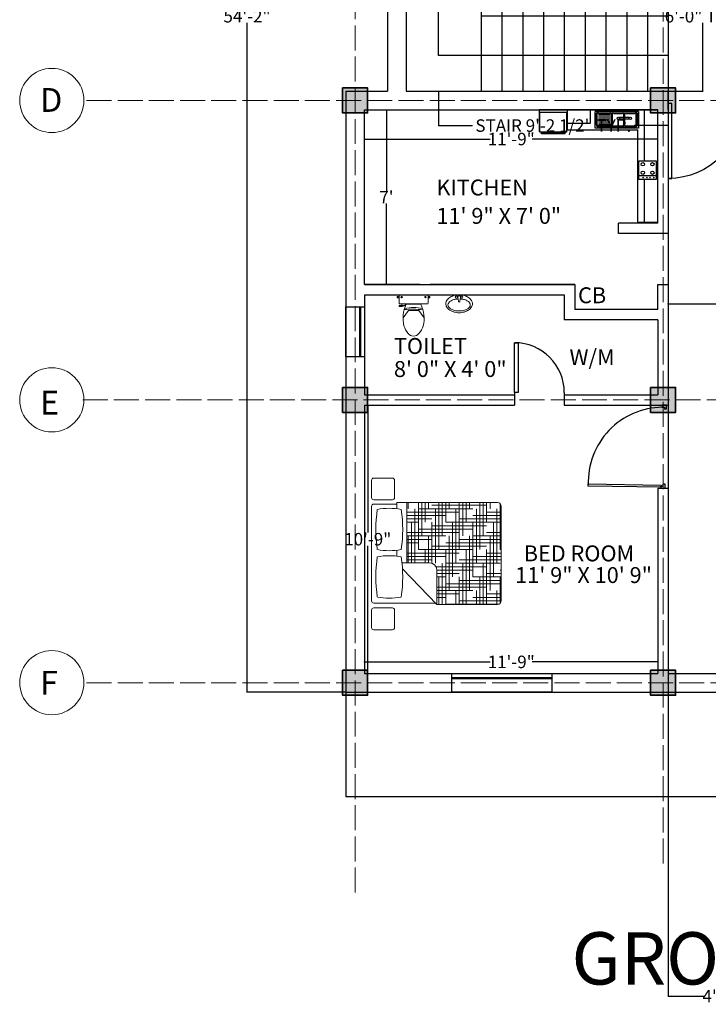
# Model space of a CAD drawing. Units: inches. Extents: x -113 to 5399, y -1393 to 3302.
# Tile 2 of 40: x 737 to 1068, y -14 to 460. Entities that reach past the tile are written whole.
import ezdxf

# ---------------------------------------------------------------- set-up
doc = ezdxf.new("R2010")
doc.units = ezdxf.units.IN
doc.header["$MEASUREMENT"] = 0
doc.linetypes.add('ACAD_ISO02W100', pattern=[15, 12, -3])
for name, color, linetype, lineweight in [('A-ANNO-DIMS', 254, 'Continuous', 18), ('A-ANNO-TEXT', 7, 'Continuous', 25), ('A-AREA-IDEN', 4, 'Continuous', 18), ('A-COLS', 7, 'Continuous', 35), ('A-FLOR-CASE', 8, 'Continuous', 18), ('A-FLOR-FIXT', 8, 'Continuous', 18), ('A-GRID-IDEN', 7, 'Continuous', 18), ('doors', 2, 'Continuous', 25), ('DT TEXT', 4, 'Continuous', 18), ('furniture', 131, 'Continuous', 18), ('GRIDS', 7, 'ACAD_ISO02W100', 13), ('stairs', 210, 'Continuous', 25), ('walls', 1, 'Continuous', 25), ('windows', 3, 'Continuous', 25)]:
    doc.layers.add(name, color=color, linetype=linetype, lineweight=lineweight)
doc.layers.add('TEFRIŞ', color=11, linetype='Continuous')
doc.styles.get("Standard").update_dxf_attribs({"font": 'arial.ttf'})
doc.dimstyles.get("Standard").update_dxf_attribs({"dimtxt": 6, "dimasz": 0.18, "dimexe": 0.18, "dimexo": 0.0625, "dimgap": 0.09, "dimtad": 0, "dimtih": 1, "dimtoh": 1, "dimdec": 1, "dimzin": 0, "dimdsep": 46, "dimlunit": 4, "dimtxsty": 'Standard', "dimblk": 'ARCHTICK', "dimcen": 0.09, "dimadec": 0, "dimazin": 0, "dimtfac": 1, "dimtdec": 1, "dimtofl": 0, "dimtmove": 0, "dimatfit": 3, "dimfxl": 1, "dimtolj": 1, "dimtzin": 0, "dimarcsym": 0})

# ---------------------------------------------------------------- blocks, each defined once
blk = doc.blocks.new('*U2')
for p, q in [((0, 0), (0, -6)), ((24, 0), (24, -6))]:
    blk.add_line(p, q)
blk.add_lwpolyline([(0, 0), (0, 24), (1.75, 24), (1.75, 0)], close=True)
blk.add_arc((0, 0), 24, 0, 90)
blk = doc.blocks.new('*U3')
for p, q in [((0, 0), (0, -6)), ((36, 0), (36, -6))]:
    blk.add_line(p, q)
blk.add_lwpolyline([(0, 0), (0, 36), (1.75, 36), (1.75, 0)], close=True)
blk.add_arc((0, 0), 36, 0, 90)
blk = doc.blocks.new('*X4')
at = {"color": 0}
for p, q in [((4.359, 18.562), (4.359, 18.646)), ((4.453, 17.817), (4.453, 18.562)), ((4.5, 18), (4.5, 18.646)), ((4.5, 18.562), (5.25, 18.562)), ((4.547, 18.188), (4.547, 18.646)), ((4.594, 18.375), (4.594, 18.646)), ((4.641, 18.562), (4.641, 18.646)), ((4.687, 18.609), (5.437, 18.609)), ((4.734, 17.812), (4.734, 18.562)), ((4.781, 18), (4.781, 18.646)), ((4.828, 18.188), (4.828, 18.646)), ((4.875, 18.375), (4.875, 18.646)), ((4.922, 18.562), (4.922, 18.646)), ((5.016, 17.812), (5.016, 18.562)), ((5.062, 18), (5.062, 18.646)), ((5.109, 18.188), (5.109, 18.646)), ((5.156, 18.375), (5.156, 18.646)), ((5.203, 18.562), (5.203, 18.646)), ((5.297, 17.812), (5.297, 18.562)), ((5.344, 18), (5.344, 18.646)), ((5.391, 18.188), (5.391, 18.646)), ((5.437, 18.375), (5.437, 18.646)), ((5.484, 18.562), (5.484, 18.646)), ((5.578, 17.812), (5.578, 18.562)), ((5.625, 18), (5.625, 18.629)), ((5.625, 18.562), (5.637, 18.562)), ((4.34, 18.516), (5.062, 18.516)), ((4.34, 18.469), (4.875, 18.469)), ((4.34, 18.422), (4.687, 18.422)), ((5.062, 18.422), (5.637, 18.422)), ((5.25, 18.469), (5.637, 18.469)), ((5.437, 18.516), (5.637, 18.516)), ((4.34, 18.375), (4.5, 18.375)), ((4.406, 17.817), (4.406, 18.375)), ((4.5, 18.281), (5.25, 18.281)), ((4.687, 18.328), (5.437, 18.328)), ((4.687, 17.811), (4.687, 18.375)), ((4.875, 18.375), (5.625, 18.375)), ((4.969, 17.625), (4.969, 18.375)), ((5.25, 17.625), (5.25, 18.375)), ((5.531, 17.625), (5.531, 18.375)), ((5.625, 18.281), (5.637, 18.281)), ((4.34, 18.234), (5.062, 18.234)), ((4.34, 18.188), (4.875, 18.188)), ((4.34, 18.141), (4.687, 18.141)), ((4.359, 17.817), (4.359, 18.188)), ((4.641, 17.817), (4.641, 18.188)), ((4.922, 17.438), (4.922, 18.188)), ((5.062, 18.141), (5.637, 18.141)), ((5.203, 17.438), (5.203, 18.188)), ((5.25, 18.188), (5.637, 18.188)), ((5.437, 18.234), (5.637, 18.234)), ((5.484, 17.438), (5.484, 18.188)), ((4.34, 18.094), (4.5, 18.094)), ((4.5, 18), (5.25, 18)), ((4.594, 17.817), (4.594, 18)), ((4.687, 18.047), (5.437, 18.047)), ((4.875, 18.094), (5.625, 18.094)), ((4.875, 17.25), (4.875, 18)), ((5.156, 17.25), (5.156, 18)), ((5.437, 17.25), (5.437, 18)), ((5.625, 18), (5.637, 18)), ((4.34, 17.953), (5.062, 17.953)), ((4.34, 17.906), (4.875, 17.906)), ((4.34, 17.859), (4.687, 17.859)), ((5.062, 17.859), (5.637, 17.859)), ((5.25, 17.906), (5.637, 17.906)), ((5.437, 17.953), (5.637, 17.953)), ((4.742, 17.766), (5.437, 17.766)), ((4.755, 17.719), (5.25, 17.719)), ((4.828, 17.246), (4.828, 17.812)), ((4.875, 17.812), (5.625, 17.812)), ((5.109, 17.246), (5.109, 17.812)), ((5.391, 17.246), (5.391, 17.812)), ((5.625, 17.719), (5.637, 17.719)), ((4.755, 17.672), (5.062, 17.672)), ((4.755, 17.625), (4.875, 17.625)), ((4.781, 17.246), (4.781, 17.625)), ((5.062, 17.246), (5.062, 17.625)), ((5.062, 17.578), (5.637, 17.578)), ((5.25, 17.625), (5.637, 17.625)), ((5.344, 17.246), (5.344, 17.625)), ((5.437, 17.672), (5.637, 17.672)), ((5.625, 17.263), (5.625, 17.625)), ((4.755, 17.484), (5.437, 17.484)), ((4.875, 17.531), (5.625, 17.531)), ((4.755, 17.438), (5.25, 17.438)), ((4.755, 17.391), (5.062, 17.391)), ((4.755, 17.344), (4.875, 17.344)), ((5.016, 17.246), (5.016, 17.438)), ((5.25, 17.344), (5.637, 17.344)), ((5.297, 17.246), (5.297, 17.438)), ((5.437, 17.391), (5.637, 17.391)), ((5.578, 17.246), (5.578, 17.438)), ((5.625, 17.438), (5.637, 17.438)), ((4.875, 17.25), (5.608, 17.25)), ((4.969, 17.246), (4.969, 17.25)), ((5.062, 17.297), (5.637, 17.297)), ((5.25, 17.246), (5.25, 17.25)), ((5.531, 17.246), (5.531, 17.25))]:
    blk.add_line(p, q, dxfattribs=at)
blk = doc.blocks.new('MAT-P01')
for p, q in [((-0.021, 0.816), (-0.021, 0.56)), ((0.009, 0.846), (0.247, 0.846)), ((0.277, 0.816), (0.277, 0.56)), ((0.344, 0.816), (0.344, -0.032)), ((0.374, 0.846), (1.674, 0.846)), ((1.704, 0.816), (1.704, 0.5)), ((1.762, 0.816), (1.762, 0.56)), ((1.792, 0.846), (2.031, 0.846)), ((2.061, 0.816), (2.061, 0.56)), ((0.009, 0.53), (0.247, 0.53)), ((0.815, 0.423), (0.324, -0.051)), ((0.895, 0.429), (0.895, 0.049)), ((0.988, 0.5), (1.069, 0.5)), ((1.639, 0.5), (1.724, 0.5)), ((1.724, 0.5), (1.724, -0.884)), ((1.792, 0.53), (2.031, 0.53)), ((0.895, 0.364), (1.724, 0.364)), ((0.895, 0.364), (0.895, 0.049)), ((0.895, 0.364), (1.724, 0.364)), ((1.724, 0.364), (1.724, -0.884)), ((0.324, -0.051), (0.795, -0.051)), ((0.324, -0.051), (0.324, -0.884)), ((0.374, -0.934), (1.674, -0.934))]:
    blk.add_line(p, q)
for centre, radius, start, end in [((0.009, 0.816), 0.03, 90, 180), ((0.247, 0.816), 0.03, 0, 90), ((0.374, 0.816), 0.03, 90, 180), ((1.674, 0.816), 0.03, 0, 90), ((1.792, 0.816), 0.03, 90, 180), ((2.031, 0.816), 0.03, 0, 90), ((1.225, 0.603), 0.814, 168.373, 191.627), ((0.703, -1.144), 1.931, 81.8162, 98.1838), ((0.181, 0.603), 0.814, 348.373, 11.627), ((1.877, 0.603), 0.814, 168.373, 191.627), ((1.354, -1.144), 1.931, 81.8162, 98.1838), ((0.832, 0.603), 0.814, 348.373, 11.627), ((0.009, 0.56), 0.03, 180, 270), ((0.247, 0.56), 0.03, 270, 0), ((1.792, 0.56), 0.03, 180, 270), ((2.031, 0.56), 0.03, 270, 0), ((0.703, 2.35), 1.931, 261.8162, 278.1838), ((1.354, 2.35), 1.931, 261.8162, 278.1838), ((0.795, 0.049), 0.1, 270, 0), ((0.374, -0.884), 0.05, 180, 270), ((1.674, -0.884), 0.05, 270, 0)]:
    blk.add_arc(centre, radius, start, end)
at = {"rotation": 270}
blk.add_blockref('*X4', (-16.922, 4.704), dxfattribs=at)
blk = doc.blocks.new('A$C008029BD')
at = {"layer": 'TEFRIŞ', "ltscale": 0.05}
for p, q in [((0, 0), (0, -3.55)), ((3.37, 0), (0, 0)), ((3.37, 0), (3.37, -0.6)), ((1.522, -0.4), (0, -0.4)), ((0.05, -0.581), (0.05, -1.869)), ((0.05, -0.581), (0.55, -0.581)), ((0.55, -0.581), (0.55, -1.869)), ((3.37, -0.4), (2.083, -0.4)), ((0.086, -1.773), (0.086, -0.677)), ((0.096, -0.617), (0.454, -0.617)), ((0.099, -0.659), (0.457, -0.659)), ((0.113, -0.954), (0.113, -0.695)), ((0.23, -0.846), (0.229, -0.967)), ((0.28, -0.846), (0.277, -1.158)), ((0.493, -0.695), (0.493, -0.954)), ((0.514, -0.677), (0.514, -1.773)), ((0.6, -2.71), (0.6, -0.6)), ((3.37, -0.6), (0.6, -0.6)), ((0.096, -1.024), (0.454, -1.024)), ((0.457, -0.99), (0.099, -0.99)), ((0.11, -1.319), (0.11, -1.06)), ((0.228, -1.02), (0.227, -1.159)), ((0.49, -1.06), (0.49, -1.319)), ((0.454, -1.355), (0.096, -1.355)), ((0.096, -1.391), (0.454, -1.391)), ((0.11, -1.773), (0.11, -1.427)), ((0.154, -1.773), (0.154, -1.427)), ((0.214, -1.773), (0.214, -1.427)), ((0.274, -1.773), (0.274, -1.427)), ((0.334, -1.773), (0.334, -1.427)), ((0.39, -1.773), (0.39, -1.427)), ((0.444, -1.773), (0.444, -1.427)), ((0.49, -1.427), (0.49, -1.773)), ((0, -2.025), (0.4, -2.025)), ((0.55, -1.869), (0.05, -1.869)), ((0.454, -1.809), (0.096, -1.809)), ((0.454, -1.833), (0.096, -1.833)), ((0.4, -2.71), (0.4, -2.025)), ((0, -2.71), (0.6, -2.71)), ((0, -3.55), (0.65, -3.55))]:
    blk.add_line(p, q, dxfattribs=at)
at = {"layer": 'TEFRIŞ'}
blk.add_line((1.969, -0.05), (1.969, -0.572), dxfattribs=at)
at = {"layer": 'TEFRIŞ', "ltscale": 0.05}
for points in [[(1.522, -0.05), (2.083, -0.05), (2.083, -0.572), (1.522, -0.572)], [(0.67, -2.73), (0.67, -3.53), (0.07, -3.53), (0.07, -2.73)], [(0.72, -2.78), (0.72, -3.48), (0.67, -3.48), (0.67, -2.78)]]:
    blk.add_lwpolyline(points, close=True, dxfattribs=at)
at = {"layer": 'TEFRIŞ', "const_width": 0.025}
for points in [[(2.014, -0.123, 1), (2.039, -0.123, 1)], [(2.014, -0.236, 1), (2.039, -0.236, 1)], [(2.014, -0.327, 1), (2.039, -0.327, 1)], [(2.014, -0.44, 1), (2.039, -0.44, 1)]]:
    blk.add_lwpolyline(points, format="xyb", close=True, dxfattribs=at)
at = {"layer": 'TEFRIŞ', "ltscale": 0.05}
for centre, radius in [((1.628, -0.164), 0.0505), ((1.628, -0.45), 0.0505), ((0.255, -0.82), 0.036), ((0.252, -1.184), 0.036)]:
    blk.add_circle(centre, radius, dxfattribs=at)
at = {"layer": 'TEFRIŞ'}
for centre in [(1.88, -0.164), (1.88, -0.45)]:
    blk.add_circle(centre, 0.0505, dxfattribs=at)
at = {"layer": 'TEFRIŞ', "ltscale": 0.05}
for centre, radius, start, end in [((0.108, -0.649), 0.0351, 110.4976, 230.5777), ((0.118, -0.673), 0.023, 143.9853, 258.5157), ((0.454, -0.677), 0.06, 0, 90), ((0.457, -0.695), 0.036, 0, 90), ((0.115, -1.038), 0.023, 143.9853, 258.5157), ((0.118, -0.976), 0.023, 101.4843, 216.0147), ((0.454, -1.06), 0.036, 0, 90), ((0.457, -0.954), 0.036, 270, 0), ((0.115, -1.341), 0.023, 101.4843, 216.0147), ((0.115, -1.405), 0.023, 143.9853, 258.5157), ((0.454, -1.319), 0.036, 270, 0), ((0.454, -1.427), 0.036, 0, 90), ((0.108, -1.801), 0.0351, 129.4223, 249.5024), ((0.115, -1.796), 0.023, 101.4843, 216.0147), ((0.454, -1.773), 0.06, 270, 0), ((0.454, -1.773), 0.036, 270, 0)]:
    blk.add_arc(centre, radius, start, end, dxfattribs=at)
blk = doc.blocks.new('toilet-3')
at = {"color": 0, "linetype": 'ByBlock'}
for p, q in [((-0.281, -0.05), (-0.281, -0.069)), ((-0.281, -0.05), (-0.261, -0.05)), ((-0.281, -0.069), (-0.261, -0.069)), ((-0.261, -0.047), (-0.261, -0.072)), ((-0.261, -0.047), (-0.251, -0.047)), ((-0.261, -0.072), (-0.251, -0.072)), ((-0.251, -0.047), (-0.251, -0.072)), ((-0.25, -0.03), (-0.25, -0.165)), ((0.24, -0.02), (-0.24, -0.02)), ((0.25, -0.03), (0.25, -0.165)), ((0.261, -0.047), (0.251, -0.047)), ((0.251, -0.047), (0.251, -0.072)), ((0.261, -0.072), (0.251, -0.072)), ((0.261, -0.047), (0.261, -0.072)), ((0.281, -0.05), (0.261, -0.05)), ((0.281, -0.069), (0.261, -0.069)), ((0.281, -0.05), (0.281, -0.069)), ((-0.144, -0.2), (-0.25, -0.2)), ((-0.25, -0.2), (-0.25, -0.222)), ((-0.198, -0.222), (-0.25, -0.222)), ((0.24, -0.175), (-0.24, -0.175)), ((-0.202, -0.2), (-0.202, -0.175)), ((-0.198, -0.222), (-0.16, -0.207)), ((-0.089, -0.287), (-0.18, -0.415)), ((-0.16, -0.207), (-0.16, -0.2)), ((-0.144, -0.2), (-0.144, -0.175)), ((0.125, -0.182), (-0.125, -0.182)), ((0.089, -0.287), (-0.089, -0.287)), ((0.089, -0.287), (0.18, -0.415))]:
    blk.add_line(p, q, dxfattribs=at)
for centre in [(-0.205, -0.059), (0.205, -0.059)]:
    blk.add_circle(centre, 0.0125, dxfattribs=at)
for centre, radius, start, end in [((-0.24, -0.03), 0.01, 90, 180), ((-0.24, -0.165), 0.01, 180, 270), ((0.24, -0.03), 0.01, 0, 90), ((0.24, -0.165), 0.01, 270, 0), ((0.376, -0.424), 0.557, 154.2321, 193.6755), ((-0.013, -1.787), 1.521, 83.4552, 95.5271), ((-0.005, -0.896), 0.659, 75.9276, 103.0204), ((-0.376, -0.424), 0.557, 346.3245, 25.7679), ((0.262, -0.406), 0.452, 199.2942, 217.2549), ((-0.265, -0.4), 0.457, 322.2382, 340.1051), ((-0.001, -0.609), 0.12, 216.3794, 323.6206)]:
    blk.add_arc(centre, radius, start, end, dxfattribs=at)
blk = doc.blocks.new('wash-6')
at = {"color": 0, "linetype": 'ByBlock'}
for p, q in [((-0.036, -0.063), (-0.021, -0.18)), ((0.036, -0.063), (0.021, -0.18))]:
    blk.add_line(p, q, dxfattribs=at)
for centre, radius in [((-0.075, -0.062), 0.0325), ((-0.075, -0.062), 0.0263), ((0.075, -0.062), 0.0325), ((0.075, -0.062), 0.0263)]:
    blk.add_circle(centre, radius, dxfattribs=at)
for centre, radius, start, end in [((0, -0.56), 0.56, 90, 105.4371), ((-0.204, -0.25), 0.17, 148.1465, 180), ((-0.204, -0.25), 0.17, 180, 211.8535), ((-0.107, -0.311), 0.285, 123.6901, 148.1465), ((-0.217, -0.282), 0.0954, 142.5096, 180), ((-0.114, -0.361), 0.225, 118.369, 142.5096), ((-0.042, -0.407), 0.401, 105.4371, 123.6901), ((-0.045, -0.488), 0.37, 102.6081, 118.369), ((0, -0.69), 0.576, 92.9466, 102.6081), ((0, -0.063), 0.0361, 0, 180), ((0, -0.18), 0.0215, 180, 0), ((0, -0.56), 0.56, 74.5629, 90), ((0, -0.69), 0.576, 77.3919, 87.0534), ((0.045, -0.488), 0.37, 61.631, 77.3919), ((0.042, -0.407), 0.401, 56.3099, 74.5629), ((0.114, -0.361), 0.225, 37.4904, 61.631), ((0.107, -0.311), 0.285, 31.8535, 56.3099), ((0.217, -0.282), 0.0954, 0, 37.4904), ((0.204, -0.25), 0.17, 0, 31.8535), ((0.204, -0.25), 0.17, 328.1465, 0), ((-0.107, -0.189), 0.285, 211.8535, 236.3099), ((-0.217, -0.282), 0.0954, 180, 217.4904), ((-0.114, -0.203), 0.225, 217.4904, 241.631), ((-0.042, -0.092), 0.401, 236.3099, 254.5629), ((-0.045, -0.076), 0.37, 241.631, 257.3919), ((0, 0.06), 0.56, 254.5629, 270), ((0, 0.125), 0.576, 257.3919, 270), ((0, 0.125), 0.576, 270, 282.6081), ((0, 0.06), 0.56, 270, 285.4371), ((0.045, -0.076), 0.37, 282.6081, 298.369), ((0.042, -0.092), 0.401, 285.4371, 303.6901), ((0.114, -0.203), 0.225, 298.369, 322.5096), ((0.107, -0.189), 0.285, 303.6901, 328.1465), ((0.217, -0.282), 0.0954, 322.5096, 0)]:
    blk.add_arc(centre, radius, start, end, dxfattribs=at)
blk = doc.blocks.new('_ArchTick')
at = {"color": 0, "linetype": 'ByBlock', "const_width": 0.15}
blk.add_lwpolyline([(-0.5, -0.5), (0.5, 0.5)], dxfattribs=at)
blk = doc.blocks.new('*D21')
at = {"layer": 'A-ANNO-DIMS', "color": 0, "lineweight": -2, "transparency": 16777216}
for p, q in [((894.23, 136.47), (894.23, 86.09)), ((1327.23, 136.47), (1327.23, 86.09)), ((894.23, 86.27), (1100.34, 86.27)), ((1327.23, 86.27), (1121.12, 86.27))]:
    blk.add_line(p, q, dxfattribs=at)
at = {"layer": 'Defpoints', "color": 0, "transparency": 16777216}
for p in [(894.23, 136.53), (1327.23, 136.53), (1327.23, 86.27)]:
    blk.add_point(p, dxfattribs=at)
at = {"layer": 'A-ANNO-DIMS', "color": 0, "lineweight": -2, "transparency": 16777216, "xscale": 0.18, "yscale": 0.18, "zscale": 0.18, "rotation": 180}
blk.add_blockref('_ArchTick', (894.23, 86.27), dxfattribs=at)
at = {"layer": 'A-ANNO-DIMS', "color": 0, "lineweight": -2, "transparency": 16777216, "xscale": 0.18, "yscale": 0.18, "zscale": 0.18}
blk.add_blockref('_ArchTick', (1327.23, 86.27), dxfattribs=at)
at = {"layer": 'A-ANNO-DIMS', "color": 0, "transparency": 16777216, "insert": (1110.73, 86.27), "char_height": 6, "attachment_point": 5}
blk.add_mtext('\\A1;36\'-1"', dxfattribs=at)
blk = doc.blocks.new('*D22')
at = {"layer": 'A-ANNO-DIMS', "color": 0, "lineweight": -2, "transparency": 16777216}
for p, q in [((894.17, 786.53), (846.52, 786.53)), ((846.7, 786.53), (846.7, 464.69)), ((846.7, 136.53), (846.7, 458.38)), ((894.17, 136.53), (846.52, 136.53))]:
    blk.add_line(p, q, dxfattribs=at)
at = {"layer": 'Defpoints', "color": 0, "transparency": 16777216}
for p in [(894.23, 786.53), (846.7, 136.53), (894.23, 136.53)]:
    blk.add_point(p, dxfattribs=at)
at = {"layer": 'A-ANNO-DIMS', "color": 0, "lineweight": -2, "transparency": 16777216, "xscale": 0.18, "yscale": 0.18, "zscale": 0.18}
for p, rotation in [((846.7, 786.53), 90), ((846.7, 136.53), 270)]:
    blk.add_blockref('_ArchTick', p, dxfattribs=dict(at, rotation=rotation))
at = {"layer": 'A-ANNO-DIMS', "color": 0, "transparency": 16777216, "insert": (846.7, 461.53), "char_height": 6, "attachment_point": 5}
blk.add_mtext('\\A1;54\'-2"', dxfattribs=at)
blk = doc.blocks.new('*D28')
at = {"layer": 'A-ANNO-DIMS', "color": 0, "lineweight": -2, "transparency": 16777216}
for p, q in [((1049.23, 323.09), (1049.23, 323.4)), ((1049.23, 323.22), (1110.33, 323.22)), ((1181.23, 323.22), (1120.13, 323.22)), ((1181.23, 323.09), (1181.23, 323.4))]:
    blk.add_line(p, q, dxfattribs=at)
at = {"layer": 'Defpoints', "color": 0, "transparency": 16777216}
for p in [(1049.23, 323.22), (1049.23, 323.03), (1181.23, 323.03)]:
    blk.add_point(p, dxfattribs=at)
at = {"layer": 'A-ANNO-DIMS', "color": 0, "lineweight": -2, "transparency": 16777216, "xscale": 0.18, "yscale": 0.18, "zscale": 0.18, "rotation": 180}
blk.add_blockref('_ArchTick', (1049.23, 323.22), dxfattribs=at)
at = {"layer": 'A-ANNO-DIMS', "color": 0, "lineweight": -2, "transparency": 16777216, "xscale": 0.18, "yscale": 0.18, "zscale": 0.18}
blk.add_blockref('_ArchTick', (1181.23, 323.22), dxfattribs=at)
at = {"layer": 'A-ANNO-DIMS', "color": 0, "transparency": 16777216, "insert": (1115.23, 323.22), "char_height": 6, "attachment_point": 5}
blk.add_mtext("\\A1;11'", dxfattribs=at)
blk = doc.blocks.new('*D33')
at = {"layer": 'A-ANNO-DIMS', "color": 0, "lineweight": -2, "transparency": 16777216}
for p, q in [((912.66, 416.53), (913.9, 416.53)), ((913.72, 416.53), (913.72, 377.62)), ((913.72, 332.53), (913.72, 371.44)), ((912.66, 332.53), (913.9, 332.53))]:
    blk.add_line(p, q, dxfattribs=at)
at = {"layer": 'Defpoints', "color": 0, "transparency": 16777216}
for p in [(912.6, 416.53), (912.6, 332.53), (913.72, 332.53)]:
    blk.add_point(p, dxfattribs=at)
at = {"layer": 'A-ANNO-DIMS', "color": 0, "lineweight": -2, "transparency": 16777216, "xscale": 0.18, "yscale": 0.18, "zscale": 0.18}
for p, rotation in [((913.72, 416.53), 90), ((913.72, 332.53), 270)]:
    blk.add_blockref('_ArchTick', p, dxfattribs=dict(at, rotation=rotation))
at = {"layer": 'A-ANNO-DIMS', "color": 0, "transparency": 16777216, "insert": (913.72, 374.53), "char_height": 6, "attachment_point": 5}
blk.add_mtext("\\A1;7'", dxfattribs=at)
blk = doc.blocks.new('*D34')
at = {"layer": 'A-ANNO-DIMS', "color": 0, "lineweight": -2, "transparency": 16777216}
for p, q in [((903.23, 402.53), (903.23, 402.64)), ((1044.23, 402.53), (1044.23, 402.64)), ((903.23, 402.46), (963.62, 402.46)), ((1044.23, 402.46), (983.84, 402.46))]:
    blk.add_line(p, q, dxfattribs=at)
at = {"layer": 'Defpoints', "color": 0, "transparency": 16777216}
for p in [(903.23, 402.46), (1044.23, 402.46), (1044.23, 402.46)]:
    blk.add_point(p, dxfattribs=at)
at = {"layer": 'A-ANNO-DIMS', "color": 0, "lineweight": -2, "transparency": 16777216, "xscale": 0.18, "yscale": 0.18, "zscale": 0.18, "rotation": 180}
blk.add_blockref('_ArchTick', (903.23, 402.46), dxfattribs=at)
at = {"layer": 'A-ANNO-DIMS', "color": 0, "lineweight": -2, "transparency": 16777216, "xscale": 0.18, "yscale": 0.18, "zscale": 0.18}
blk.add_blockref('_ArchTick', (1044.23, 402.46), dxfattribs=at)
at = {"layer": 'A-ANNO-DIMS', "color": 0, "transparency": 16777216, "insert": (973.73, 402.46), "char_height": 6, "attachment_point": 5}
blk.add_mtext('\\A1;11\'-9"', dxfattribs=at)
blk = doc.blocks.new('*D35')
at = {"layer": 'A-ANNO-DIMS', "color": 0, "lineweight": -2, "transparency": 16777216}
for p, q in [((904.22, 274.53), (904.94, 274.53)), ((904.76, 274.53), (904.76, 213.19)), ((904.76, 145.53), (904.76, 206.88)), ((904.22, 145.53), (904.94, 145.53))]:
    blk.add_line(p, q, dxfattribs=at)
at = {"layer": 'Defpoints', "color": 0, "transparency": 16777216}
for p in [(904.15, 274.53), (904.15, 145.53), (904.76, 145.53)]:
    blk.add_point(p, dxfattribs=at)
at = {"layer": 'A-ANNO-DIMS', "color": 0, "lineweight": -2, "transparency": 16777216, "xscale": 0.18, "yscale": 0.18, "zscale": 0.18}
for p, rotation in [((904.76, 274.53), 90), ((904.76, 145.53), 270)]:
    blk.add_blockref('_ArchTick', p, dxfattribs=dict(at, rotation=rotation))
at = {"layer": 'A-ANNO-DIMS', "color": 0, "transparency": 16777216, "insert": (904.76, 210.03), "char_height": 6, "attachment_point": 5}
blk.add_mtext('\\A1;10\'-9"', dxfattribs=at)
blk = doc.blocks.new('*D36')
at = {"layer": 'A-ANNO-DIMS', "color": 0, "lineweight": -2, "transparency": 16777216}
for p, q in [((903.23, 150.98), (903.23, 151.21)), ((903.23, 151.03), (963.62, 151.03)), ((1044.23, 151.03), (983.84, 151.03)), ((1044.23, 150.98), (1044.23, 151.21))]:
    blk.add_line(p, q, dxfattribs=at)
at = {"layer": 'Defpoints', "color": 0, "transparency": 16777216}
for p in [(903.23, 151.03), (903.23, 150.91), (1044.23, 150.91)]:
    blk.add_point(p, dxfattribs=at)
at = {"layer": 'A-ANNO-DIMS', "color": 0, "lineweight": -2, "transparency": 16777216, "xscale": 0.18, "yscale": 0.18, "zscale": 0.18, "rotation": 180}
blk.add_blockref('_ArchTick', (903.23, 151.03), dxfattribs=at)
at = {"layer": 'A-ANNO-DIMS', "color": 0, "lineweight": -2, "transparency": 16777216, "xscale": 0.18, "yscale": 0.18, "zscale": 0.18}
blk.add_blockref('_ArchTick', (1044.23, 151.03), dxfattribs=at)
at = {"layer": 'A-ANNO-DIMS', "color": 0, "transparency": 16777216, "insert": (973.73, 151.03), "char_height": 6, "attachment_point": 5}
blk.add_mtext('\\A1;11\'-9"', dxfattribs=at)
blk = doc.blocks.new('WIN-PLAN-48IN')
h = blk.add_hatch(color=256)
h.dxf.hatch_style = 1
h.paths.add_polyline_path([(48, 2.5), (0, 2.5), (0, 2), (48, 2)])
for p, q in [((0, 9), (48, 9)), ((0, 0), (0, 9)), ((48, 9), (48, 0)), ((48, 2.5), (0, 2.5)), ((48, 2), (0, 2)), ((48, 0), (0, 0))]:
    blk.add_line(p, q)
blk = doc.blocks.new('WIN-PLAN-24IN')
h = blk.add_hatch(color=256)
h.dxf.hatch_style = 1
h.paths.add_polyline_path([(6.5, 24), (6.5, 0), (7, 0), (7, 24)])
for p, q in [((0, 0), (0, 24)), ((0, 24), (9, 24)), ((6.5, 24), (6.5, 0)), ((7, 24), (7, 0)), ((9, 24), (9, 0)), ((9, 0), (0, 0))]:
    blk.add_line(p, q)
blk = doc.blocks.new('COLUMN-12IN-SQUARE')
h = blk.add_hatch(color=256)
h.dxf.hatch_style = 1
h.paths.add_polyline_path([(6, 6), (-6, 6), (-6, -6), (6, -6)])
blk.add_lwpolyline([(-6, 6), (6, 6), (6, -6), (-6, -6)], close=True)
blk = doc.blocks.new('STAIR-RESIDENTIAL-PLAN')
for p, q in [((20.54, 72), (20.54, 0)), ((30.54, 72), (30.54, 0)), ((40.54, 72), (40.54, 0)), ((50.54, 72), (50.54, 0)), ((60.54, 72), (60.54, 0)), ((70.54, 72), (70.54, 0)), ((80.54, 72), (80.54, 0)), ((90.54, 72), (90.54, 0)), ((100.54, 72), (100.54, 0)), ((110.54, 72), (110.54, 0)), ((110.54, 54.14), (107.61, 56.9)), ((107.61, 56.9), (107.61, 54.14)), ((0, 17.09), (0, 54.14)), ((0, 54.14), (107.61, 54.14)), ((110.54, 54.14), (107.61, 51.38)), ((107.61, 51.38), (107.61, 54.14)), ((110.54, 36), (20.54, 36)), ((110.54, 17.09), (0, 17.09))]:
    blk.add_line(p, q)
blk = doc.blocks.new('DOOR-SINGLE-36IN-PLAN')
for p, q in [((0.5, 2), (0.5, 36.98)), ((0.5, 36.98), (1.5, 36.98)), ((1.5, 36.98), (1.5, 2)), ((0, 2), (0, 0)), ((0, 2), (1.04, 2)), ((1.5, 2), (0.5, 2)), ((1.04, 2), (1.04, 0.98)), ((1.04, 0.98), (2, 0.98)), ((2, 0), (2, 0.98)), ((38.96, 0.98), (38, 0.98)), ((38, 0), (38, 0.98)), ((40, 2), (38.96, 2)), ((38.96, 2), (38.96, 0.98)), ((40, 0), (40, 2)), ((0, 0), (2, 0)), ((0, 0), (2, 0)), ((38, 0), (40, 0))]:
    blk.add_line(p, q)
blk.add_arc((2.94, 0.99), 36.04, 1.6003, 93.0893)
blk = doc.blocks.new('GRID-BUBBLE-D')
blk.add_circle((0, 0), 15.44)
blk.add_text('D', height=11.45).set_placement((-5.69, -5.49))
blk = doc.blocks.new('GRID-BUBBLE-E')
blk.add_circle((0, 0), 15.44)
blk.add_text('E', height=11.45).set_placement((-5.69, -7.06))
blk = doc.blocks.new('GRID-BUBBLE-F')
blk.add_circle((0, 0), 15.44)
blk.add_text('F', height=11.45).set_placement((-5.69, -5.75))
blk = doc.blocks.new('*D193')
at = {"layer": 'A-ANNO-DIMS', "color": 0, "lineweight": -2, "transparency": 16777216}
for p, q in [((938.69, 425.47), (938.69, 408.77)), ((1049.23, 425.47), (1049.23, 408.77)), ((938.69, 408.95), (955.1, 408.95)), ((1049.23, 408.95), (1032.82, 408.95))]:
    blk.add_line(p, q, dxfattribs=at)
at = {"layer": 'Defpoints', "color": 0, "transparency": 16777216}
for p in [(938.69, 425.53), (1049.23, 425.53), (1049.23, 408.95)]:
    blk.add_point(p, dxfattribs=at)
at = {"layer": 'A-ANNO-DIMS', "color": 0, "lineweight": -2, "transparency": 16777216, "xscale": 0.18, "yscale": 0.18, "zscale": 0.18, "rotation": 180}
blk.add_blockref('_ArchTick', (938.69, 408.95), dxfattribs=at)
at = {"layer": 'A-ANNO-DIMS', "color": 0, "lineweight": -2, "transparency": 16777216, "xscale": 0.18, "yscale": 0.18, "zscale": 0.18}
blk.add_blockref('_ArchTick', (1049.23, 408.95), dxfattribs=at)
at = {"layer": 'A-ANNO-DIMS', "color": 0, "transparency": 16777216, "insert": (993.96, 408.95), "char_height": 6, "attachment_point": 5}
blk.add_mtext('\\A1;STAIR 9\'-2 1/2" TYP.', dxfattribs=at)
blk = doc.blocks.new('*D194')
at = {"layer": 'A-ANNO-DIMS', "color": 0, "lineweight": -2, "transparency": 16777216}
for p, q in [((1049.29, 497.53), (1065.99, 497.53)), ((1065.81, 497.53), (1065.81, 464.69)), ((1065.81, 425.53), (1065.81, 458.38)), ((1049.29, 425.53), (1065.99, 425.53))]:
    blk.add_line(p, q, dxfattribs=at)
at = {"layer": 'Defpoints', "color": 0, "transparency": 16777216}
for p in [(1049.23, 497.53), (1065.81, 497.53), (1049.23, 425.53)]:
    blk.add_point(p, dxfattribs=at)
at = {"layer": 'A-ANNO-DIMS', "color": 0, "lineweight": -2, "transparency": 16777216, "xscale": 0.18, "yscale": 0.18, "zscale": 0.18}
for p, rotation in [((1065.81, 497.53), 90), ((1065.81, 425.53), 270)]:
    blk.add_blockref('_ArchTick', p, dxfattribs=dict(at, rotation=rotation))
at = {"layer": 'A-ANNO-DIMS', "color": 0, "transparency": 16777216, "insert": (1065.81, 461.53), "char_height": 6, "attachment_point": 5}
blk.add_mtext('\\A1;6\'-0" TYP.', dxfattribs=at)
blk = doc.blocks.new('*D212')
at = {"layer": 'A-ANNO-DIMS', "color": 0, "lineweight": -2, "transparency": 16777216}
for p, q in [((1049.23, 425.47), (1049.23, -9.87)), ((1100.23, 425.47), (1100.23, -9.87)), ((1049.23, -9.69), (1066.55, -9.69)), ((1100.23, -9.69), (1082.92, -9.69))]:
    blk.add_line(p, q, dxfattribs=at)
at = {"layer": 'Defpoints', "color": 0, "transparency": 16777216}
for p in [(1049.23, 425.53), (1100.23, 425.53), (1100.23, -9.69)]:
    blk.add_point(p, dxfattribs=at)
at = {"layer": 'A-ANNO-DIMS', "color": 0, "lineweight": -2, "transparency": 16777216, "xscale": 0.18, "yscale": 0.18, "zscale": 0.18, "rotation": 180}
blk.add_blockref('_ArchTick', (1049.23, -9.69), dxfattribs=at)
at = {"layer": 'A-ANNO-DIMS', "color": 0, "lineweight": -2, "transparency": 16777216, "xscale": 0.18, "yscale": 0.18, "zscale": 0.18}
blk.add_blockref('_ArchTick', (1100.23, -9.69), dxfattribs=at)
at = {"layer": 'A-ANNO-DIMS', "color": 0, "transparency": 16777216, "insert": (1074.73, -9.69), "char_height": 6, "attachment_point": 5}
blk.add_mtext('\\A1;4\'-3"', dxfattribs=at)

msp = doc.modelspace()

# ---------------------------------------------------------------- linework, layer by layer
at = {"layer": 'GRIDS'}
for p, q in [((898.65, 922.09), (898.65, 39.31)), ((1046.73, 54.04), (1046.73, 921.39)), ((1426.54, 421.03), (768.3, 421.03)), ((767.75, 277.03), (1426.54, 277.03)), ((1426.54, 141.03), (768.3, 141.03))]:
    msp.add_line(p, q, dxfattribs=at)
at = {"layer": 'walls'}
for p, q in [((914.23, 497.53), (914.23, 425.53)), ((923.23, 497.53), (923.23, 425.53)), ((894.23, 425.53), (894.23, 136.53)), ((894.23, 425.53), (914.23, 425.53)), ((923.23, 425.53), (1049.23, 425.53)), ((1049.23, 416.53), (1049.23, 425.53)), ((903.23, 416.53), (987.08, 416.53)), ((903.23, 332.53), (903.23, 416.53)), ((934.73, 416.53), (1044.23, 416.53)), ((1044.23, 362.03), (1044.23, 416.53)), ((1049.23, 416.53), (1049.23, 357.03)), ((1044.23, 362.03), (1025.23, 362.03)), ((1025.23, 357.03), (1025.23, 362.03)), ((1049.23, 357.03), (1025.23, 357.03)), ((929.73, 332.53), (903.23, 332.53)), ((903.23, 332.53), (929.73, 332.53)), ((929.73, 332.53), (934.73, 332.53)), ((1004.23, 332.53), (934.73, 332.53)), ((934.73, 332.53), (1004.23, 332.53)), ((1004.23, 332.53), (1004.23, 320.53)), ((1044.23, 320.53), (1044.23, 332.53)), ((1044.23, 332.53), (1049.23, 332.53)), ((1049.23, 332.53), (1049.23, 274.53)), ((903.23, 327.53), (903.23, 279.53)), ((903.23, 327.53), (999.23, 327.53)), ((903.23, 327.53), (999.23, 327.53)), ((999.23, 327.53), (999.23, 315.53)), ((1044.23, 320.53), (1004.23, 320.53)), ((1044.23, 315.53), (999.23, 315.53)), ((1044.23, 315.53), (1044.23, 279.53)), ((903.23, 279.53), (975.23, 279.53)), ((975.23, 279.53), (975.23, 274.53)), ((999.23, 280.53), (999.23, 274.53)), ((999.23, 279.53), (1044.23, 279.53)), ((903.23, 274.53), (903.23, 145.53)), ((903.23, 274.53), (975.23, 274.53)), ((999.23, 274.53), (1044.23, 274.53)), ((1044.23, 274.53), (1049.23, 274.53)), ((1044.23, 234.53), (1044.23, 145.53)), ((1044.23, 234.53), (1049.23, 234.53)), ((1049.23, 234.53), (1049.23, 145.53)), ((903.23, 145.53), (1044.23, 145.53)), ((1049.23, 145.53), (1091.23, 145.53)), ((894.23, 136.53), (1091.23, 136.53))]:
    msp.add_line(p, q, dxfattribs=at)

# ---------------------------------------------------------------- block references
at = {"layer": 'A-COLS'}
for p in [(898.65, 421.03), (1046.73, 421.03), (898.65, 277.03), (1046.73, 277.03), (898.65, 141.03), (1046.73, 141.03)]:
    msp.add_blockref('COLUMN-12IN-SQUARE', p, dxfattribs=at)
at = {"layer": 'A-FLOR-CASE', "xscale": 16.09806929200166, "yscale": 16.09806929200166, "zscale": 16.09806929200166, "rotation": 270}
msp.add_blockref('A$C008029BD', (1044.23, 416.53), dxfattribs=at)
at = {"layer": 'A-FLOR-FIXT'}
for name, p, xscale, yscale, zscale in [('toilet-3', (926.77, 328.09), 27.95492935005888, 27.95492935005888, 27.95492935005888), ('wash-6', (948.68, 327.53), 17.16666334294967, 17.16666334294967, 17.16666334294967)]:
    msp.add_blockref(name, p, dxfattribs=dict(at, xscale=xscale, yscale=yscale, zscale=zscale))
at = {"layer": 'A-GRID-IDEN'}
for name, p in [('GRID-BUBBLE-D', (752.86, 421.03)), ('GRID-BUBBLE-E', (752.86, 277.03)), ('GRID-BUBBLE-F', (752.86, 141.03))]:
    msp.add_blockref(name, p, dxfattribs=at)
at = {"layer": 'doors', "xscale": -1, "rotation": 180}
msp.add_blockref('*U3', (1049.23, 419.53), dxfattribs=at)
at = {"layer": 'doors'}
msp.add_blockref('*U2', (975.23, 280.53), dxfattribs=at)
at = {"layer": 'doors', "rotation": 89.09244041659068}
msp.add_blockref('DOOR-SINGLE-36IN-PLAN', (1047.73, 234.52), dxfattribs=at)
at = {"layer": 'furniture', "xscale": 35.02364872074636, "yscale": 35.02364872074636, "zscale": 35.02364872074636, "rotation": 90}
msp.add_blockref('MAT-P01', (936.22, 167.26), dxfattribs=at)
at = {"layer": 'stairs'}
msp.add_blockref('STAIR-RESIDENTIAL-PLAN', (938.69, 425.53), dxfattribs=at)
at = {"layer": 'windows'}
msp.add_blockref('WIN-PLAN-24IN', (894.23, 297.81), dxfattribs=at)
at = {"layer": 'windows', "rotation": 180}
msp.add_blockref('WIN-PLAN-48IN', (993.23, 145.53), dxfattribs=at)

# ---------------------------------------------------------------- texts
at = {"layer": 'A-ANNO-TEXT'}
msp.add_text('GROUND FLOOR', height=25.17, dxfattribs=at).set_placement((1002.73, -4.13))
at = {"layer": 'A-AREA-IDEN'}
for s, height, p in [('KITCHEN', 7.647, (937.75, 375.36)), ('11\' 9" X 7\' 0"', 7.6473, (937.75, 361.69)), ('TOILET', 7.647, (917.32, 299.13)), ('8\' 0" X 4\' 0"', 7.6473, (917.32, 288.04)), ('BED ROOM', 7.647, (979.74, 199.39)), ('11\' 9" X 10\' 9"', 7.6473, (975.63, 188.96))]:
    msp.add_text(s, height=height, dxfattribs=at).set_placement(p)
at = {"layer": 'DT TEXT'}
for s, p in [('CB', (1005.85, 323.51)), (' W/M', (999.39, 293.76))]:
    msp.add_text(s, height=7.647, dxfattribs=at).set_placement(p)

# ---------------------------------------------------------------- dimensions: what is measured, and where the dimension line sits
at = {"layer": 'A-ANNO-DIMS'}
for base, p1, p2, picture, middle in [((846.7, 136.53), (894.23, 786.53), (894.23, 136.53), '*D22', (846.7, 461.53)), ((913.72, 332.53), (912.6, 416.53), (912.6, 332.53), '*D33', (913.72, 374.53)), ((904.76, 145.53), (904.15, 274.53), (904.15, 145.53), '*D35', (904.76, 210.03))]:
    dim = msp.add_linear_dim(base=base, p1=p1, p2=p2, angle=90, dimstyle='Standard', override={"dimclrd": 0, "dimclre": 0, "dimclrt": 0}, dxfattribs=at)
    dim.commit()
    dim.dimension.update_dxf_attribs({"geometry": picture, "text_midpoint": middle})
dim = msp.add_linear_dim(base=(1065.81, 497.53), p1=(1049.23, 425.53), p2=(1049.23, 497.53), angle=90, text='<> TYP.', dimstyle='Standard', override={"dimdec": 1, "dimlfac": 1, "dimrnd": 0, "dimzin": 1, "dimdsep": 46, "dimlunit": 4, "dimfrac": 2}, dxfattribs=at)
dim.commit()
dim.dimension.update_dxf_attribs({"geometry": '*D194', "text_midpoint": (1065.81, 461.53)})
dim = msp.add_linear_dim(base=(1049.23, 408.95), p1=(938.69, 425.53), p2=(1049.23, 425.53), text='STAIR <> TYP.', dimstyle='Standard', override={"dimdec": 1, "dimlfac": 1, "dimrnd": 0, "dimzin": 1, "dimdsep": 46, "dimlunit": 4, "dimfrac": 2}, dxfattribs=at)
dim.commit()
dim.dimension.update_dxf_attribs({"geometry": '*D193', "text_midpoint": (993.96, 408.95)})
for base, p1, p2, override, picture, middle in [((1100.23, -9.69), (1049.23, 425.53), (1100.23, 425.53), {"dimdec": 1, "dimlfac": 1, "dimrnd": 0, "dimzin": 1, "dimdsep": 46, "dimlunit": 4, "dimfrac": 2}, '*D212', (1074.73, -9.69)), ((1044.23, 402.46), (903.23, 402.46), (1044.23, 402.46), {"dimclrd": 0, "dimclre": 0, "dimclrt": 0}, '*D34', (973.73, 402.46)), ((1049.23, 323.22), (1181.23, 323.03), (1049.23, 323.03), {"dimclrd": 0, "dimclre": 0, "dimclrt": 0}, '*D28', (1115.23, 323.22)), ((903.23, 151.03), (1044.23, 150.91), (903.23, 150.91), {"dimclrd": 0, "dimclre": 0, "dimclrt": 0}, '*D36', (973.73, 151.03)), ((1327.23, 86.27), (894.23, 136.53), (1327.23, 136.53), {"dimclrd": 0, "dimclre": 0, "dimclrt": 0}, '*D21', (1110.73, 86.27))]:
    dim = msp.add_linear_dim(base=base, p1=p1, p2=p2, dimstyle='Standard', override=override, dxfattribs=at)
    dim.commit()
    dim.dimension.update_dxf_attribs({"geometry": picture, "text_midpoint": middle})

doc.saveas('drawing.dxf')
